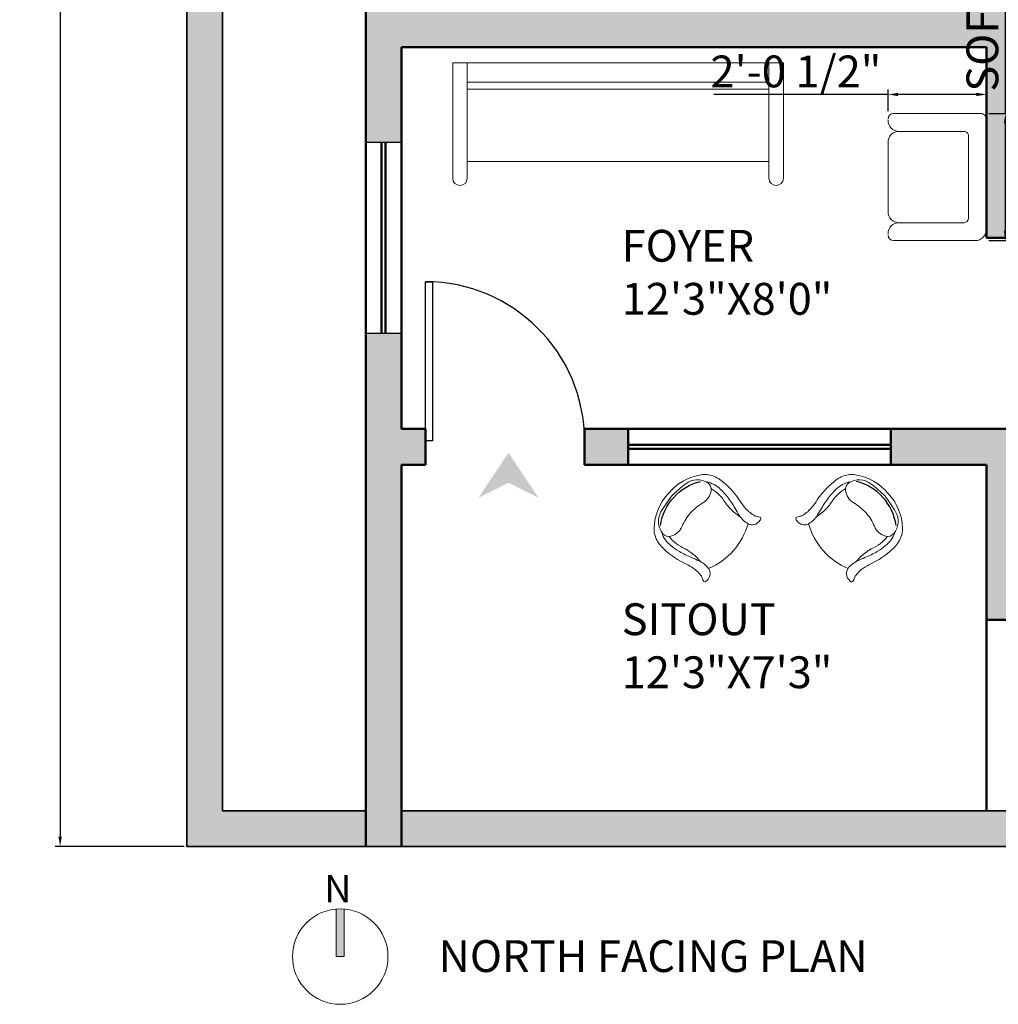
# Model space of a CAD drawing. Units: inches. Extents: x 2442 to 3851, y 589 to 2836.
# Tile 3 of 22: x 2452 to 2698, y 1362 to 1610. Entities that reach past the tile are written whole.
import ezdxf

# ---------------------------------------------------------------- set-up
doc = ezdxf.new("R2010")
doc.units = ezdxf.units.IN
for name, color, linetype, lineweight in [('A-ANNO-DIMS', 2, 'Continuous', 18), ('A-ANNO-SYMB', 1, 'Continuous', 18), ('A-ANNO-TEXT', 7, 'Continuous', 18), ('A-AREA-IDEN', 7, 'Continuous', 18), ('A-DOOR', 4, 'Continuous', 25), ('A-FURN', 8, 'Continuous', 18), ('A-GLAZ', 1, 'Continuous', 25), ('A-WALL', 7, 'Continuous', 50), ('A-WALL-PATT', 8, 'Continuous', 13), ('C-PROP', 7, 'Continuous', 35)]:
    doc.layers.add(name, color=color, linetype=linetype, lineweight=lineweight)
doc.layers.add('IFF-FURN-DETAIL', color=250, linetype='Continuous')
doc.styles.get("Standard").update_dxf_attribs({"font": 'arial.ttf'})
doc.dimstyles.new('ISO-25', dxfattribs={"dimtxt": 8, "dimasz": 2.5, "dimexe": 1.25, "dimexo": 0.625, "dimtad": 1, "dimlunit": 3, "dimtxsty": 'Standard', "dimcen": 2.5, "dimadec": 0, "dimazin": 0, "dimtfac": 1, "dimtmove": 0, "dimatfit": 3, "dimfxl": 1, "dimarcsym": 0})

# ---------------------------------------------------------------- blocks, each defined once
blk = doc.blocks.new('*U22')
for p, q in [((0, 0), (0, -6)), ((40, 0), (40, -6))]:
    blk.add_line(p, q)
blk.add_lwpolyline([(0, 0), (0, 40), (1.75, 40), (1.75, 0)], close=True)
blk.add_arc((0, 0), 40, 0, 90)
blk = doc.blocks.new('sofa-27')
at = {"color": 0, "linetype": 'ByBlock'}
for p, q in [((-0.0591, 0.0591), (-0.0591, 0.4902)), ((0.0945, 0.5198), (0.459, 0.5198)), ((0.6125, 0.0295), (0.6125, 0.4902)), ((0.0354, 0.1181), (0.0354, 0.4607)), ((0.518, 0.1181), (0.518, 0.4607)), ((0.4944, 0.0945), (0.0591, 0.0945)), ((0.583, 0), (0, 0))]:
    blk.add_line(p, q, dxfattribs=at)
for centre, radius, start, end in [((-0.0295, 0.4902), 0.0295, 90, 180), ((-0.0236, 0.4607), 0.0591, 360, 90), ((0.0945, 0.4607), 0.0591, 90, 180), ((0.459, 0.4607), 0.0591, 0, 90), ((0.5771, 0.4607), 0.0591, 90, 180), ((0.583, 0.4902), 0.0295, 0, 90), ((0.0591, 0.1181), 0.0236, 180, 270), ((0.4944, 0.1181), 0.0236, 270, 0), ((0, 0.0591), 0.0591, 180, 270), ((0.583, 0.0295), 0.0295, 270, 0)]:
    blk.add_arc(centre, radius, start, end, dxfattribs=at)
blk = doc.blocks.new('ILNG95')
for points in [[(120, 308, -0.32971), (51, 384, -0.036099), (50, 422, -0.497733), (75, 439, -0.070621), (96, 429, 0.101868), (133, 414, 0.091794), (259, 412, 0.024114), (351, 433, -0.090294), (638, 458, -0.132412), (775, 407, -0.068618), (816, 368, -0.184346), (943, 0, 1.803905)], [(120, 308, 0.138132), (244, 313, 0.001085), (325, 339, -0.034227), (462, 375, -0.033255), (567, 387, -0.137428), (727, 350, -4.561553)], [(120, 308, 0.138132), (244, 313, 0.001085), (325, 339, -0.034227), (462, 375, -0.033255), (567, 387, -0.137428), (727, 350, -4.561553)], [(235, 308, 0.064243), (394, 307, 0.04414), (433, 315, -0.118032), (643, 329, -6.296816)], [(235, 308, 0.064243), (394, 307, 0.04414), (433, 315, -0.118032), (643, 329, -6.296816)], [(639, 0, 0.078302), (612, 161, -0.233633), (633, 315, -0.28763), (710, 349, -0.317923), (875, 193, -0.032882), (900, 0, 1.140397)], [(639, 0, 0.078302), (612, 161, -0.233633), (633, 315, -0.28763), (710, 349, -0.317923), (875, 193, -0.032882), (900, 0, 1.140397)], [(120, -308, 0.32971), (51, -384, 0.036099), (50, -422, 0.497733), (75, -439, 0.070621), (96, -429, -0.101868), (133, -414, -0.091794), (259, -412, -0.024114), (351, -433, 0.090294), (638, -458, 0.132412), (775, -407, 0.068618), (816, -368, 0.184346), (943, 0, -1.803905)], [(639, 0, -0.078302), (612, -161, 0.233633), (633, -315, 0.28763), (710, -349, 0.317923), (875, -193, 0.032882), (900, 0, -1.140397)], [(639, 0, -0.078302), (612, -161, 0.233633), (633, -315, 0.28763), (710, -349, 0.317923), (875, -193, 0.032882), (900, 0, -1.140397)], [(120, -308, -0.138132), (244, -313, -0.001085), (325, -339, 0.034227), (462, -375, 0.033255), (567, -387, 0.137428), (727, -350, 4.561553)], [(120, -308, -0.138132), (244, -313, -0.001085), (325, -339, 0.034227), (462, -375, 0.033255), (567, -387, 0.137428), (727, -350, 4.561553)], [(235, -308, -0.064243), (394, -307, -0.04414), (433, -315, 0.118032), (643, -329, 6.296816)], [(235, -308, -0.064243), (394, -307, -0.04414), (433, -315, 0.118032), (643, -329, 6.296816)]]:
    blk.add_lwpolyline(points, format="xyb")
blk.add_arc((759, 1), 709, 154.3281, 205.801)
at = {"layer": 'IFF-FURN-DETAIL'}
blk.add_arc((326, -2), 549, 326.8997, 34.6691, dxfattribs=at)
blk.add_arc((326, -2), 549, 326.8997, 34.6691, dxfattribs=at)
blk = doc.blocks.new('*D32')
at = {"layer": 'A-ANNO-DIMS', "color": 0, "lineweight": -2, "transparency": 16777216}
for p, q in [((2492.97, 2001.86), (2460.53, 2001.86)), ((2461.78, 1999.36), (2461.78, 1404.36)), ((2492.97, 1401.86), (2460.53, 1401.86))]:
    blk.add_line(p, q, dxfattribs=at)
at = {"layer": 'A-ANNO-DIMS', "color": 0, "transparency": 16777216}
for points in [[(2461.36, 1999.36), (2462.2, 1999.36), (2461.78, 2001.86)], [(2461.36, 1404.36), (2462.2, 1404.36), (2461.78, 1401.86)]]:
    blk.add_solid(points, dxfattribs=at)
at = {"layer": 'Defpoints', "color": 0, "transparency": 16777216}
for p in [(2493.6, 2001.86), (2461.78, 1401.86), (2493.6, 1401.86)]:
    blk.add_point(p, dxfattribs=at)
at = {"layer": 'A-ANNO-DIMS', "color": 0, "transparency": 16777216, "insert": (2457.07, 1701.86), "char_height": 8, "attachment_point": 5, "rotation": 90}
blk.add_mtext("50'", dxfattribs=at)
blk = doc.blocks.new('SOFA-3SEAT')
for p, q in [((0, 29.02), (0, 0)), ((3.63, 0), (3.63, 29.02)), ((79.48, 29.02), (79.48, 0)), ((83.11, 29.02), (83.11, 0)), ((83.11, 0), (0, 0))]:
    blk.add_line(p, q)
for centre in [(1.81, 29.02), (81.3, 29.02)]:
    blk.add_arc(centre, 1.81, 0, 180)
blk = doc.blocks.new('NORTH-ARROW')
at = {"transparency": 33554687}
h = blk.add_hatch(color=256, dxfattribs=at)
h.dxf.hatch_style = 1
h.paths.add_polyline_path([(13, 12), (11, 12), (11, 23.96, -0.020861), (12, 24, -0.020861), (13, 23.96)])
for p, q in [((11, 24), (11, 12)), ((13, 12), (13, 23.96)), ((11, 12), (13, 12))]:
    blk.add_line(p, q)
blk.add_circle((12, 12), 12)
blk.add_text('N', height=6.9).set_placement((7.98, 25.6))
blk = doc.blocks.new('*D150')
at = {"layer": 'A-ANNO-DIMS', "color": 0, "lineweight": -2, "transparency": 16777216}
for p, q in [((2699.39, 1586.16), (2699.39, 1682.55)), ((2695.22, 1586.16), (2700.64, 1586.16)), ((2699.39, 1556.72), (2699.39, 1583.66)), ((2695.22, 1554.22), (2700.64, 1554.22))]:
    blk.add_line(p, q, dxfattribs=at)
at = {"layer": 'A-ANNO-DIMS', "color": 0, "transparency": 16777216}
for points in [[(2698.97, 1583.66), (2699.81, 1583.66), (2699.39, 1586.16)], [(2698.97, 1556.72), (2699.81, 1556.72), (2699.39, 1554.22)]]:
    blk.add_solid(points, dxfattribs=at)
at = {"layer": 'Defpoints', "color": 0, "transparency": 16777216}
for p in [(2694.6, 1586.16), (2699.39, 1586.16), (2694.6, 1554.22)]:
    blk.add_point(p, dxfattribs=at)
at = {"layer": 'A-ANNO-DIMS', "color": 0, "transparency": 16777216, "insert": (2694.63, 1635.61), "char_height": 8, "attachment_point": 5, "rotation": 90}
blk.add_mtext('SOFA CHAIR 2\'-8"', dxfattribs=at)
blk = doc.blocks.new('*D151')
at = {"layer": 'A-ANNO-DIMS', "color": 0, "lineweight": -2, "transparency": 16777216}
for p, q in [((2669.88, 1586.79), (2669.88, 1592.2)), ((2694.6, 1586.79), (2694.6, 1592.2)), ((2669.88, 1590.95), (2626.08, 1590.95)), ((2692.1, 1590.95), (2672.38, 1590.95))]:
    blk.add_line(p, q, dxfattribs=at)
at = {"layer": 'A-ANNO-DIMS', "color": 0, "transparency": 16777216}
for points in [[(2672.38, 1591.37), (2672.38, 1590.54), (2669.88, 1590.95)], [(2692.1, 1591.37), (2692.1, 1590.54), (2694.6, 1590.95)]]:
    blk.add_solid(points, dxfattribs=at)
at = {"layer": 'Defpoints', "color": 0, "transparency": 16777216}
for p in [(2669.88, 1590.95), (2669.88, 1586.16), (2694.6, 1586.16)]:
    blk.add_point(p, dxfattribs=at)
at = {"layer": 'A-ANNO-DIMS', "color": 0, "transparency": 16777216, "insert": (2646.73, 1595.71), "char_height": 8, "attachment_point": 5}
blk.add_mtext('2\'-0 1/2"', dxfattribs=at)

msp = doc.modelspace()

# ---------------------------------------------------------------- hatches: boundary and pattern name
at = {"layer": 'A-ANNO-SYMB'}
h = msp.add_hatch(color=256, dxfattribs=at)
h.dxf.hatch_style = 1
h.paths.add_polyline_path([(2574.486, 1500.868), (2566.935, 1489.543), (2574.486, 1493.318), (2582.036, 1489.543)])
at = {"layer": 'A-WALL-PATT'}
h = msp.add_hatch(color=256, dxfattribs=at)
h.dxf.hatch_style = 1
h.paths.add_polyline_path([(2502.599, 1992.864), (2719.571, 1992.864), (2719.687, 1994.649), (2720.167, 1997.319), (2721.479, 1992.864), (2726.325, 1992.864), (2727.448, 1994.93), (2729.005, 1997.153), (2728.372, 1992.864), (2728.871, 1992.864), (2730.114, 1994.505), (2731.833, 1996.09), (2730.966, 1993.206), (2730.864, 1992.864), (2771.772, 1992.864), (2771.887, 1994.649), (2772.368, 1997.319), (2773.68, 1992.864), (2778.526, 1992.864), (2779.649, 1994.93), (2781.206, 1997.153), (2780.572, 1992.864), (2781.072, 1992.864), (2782.315, 1994.505), (2784.034, 1996.09), (2783.167, 1993.206), (2783.065, 1992.864), (2821.282, 1992.864), (2821.398, 1994.649), (2821.878, 1997.319), (2823.19, 1992.864), (2828.036, 1992.864), (2829.159, 1994.93), (2830.716, 1997.153), (2830.083, 1992.864), (2830.582, 1992.864), (2831.825, 1994.505), (2833.544, 1996.09), (2832.677, 1993.206), (2832.575, 1992.864), (2869.287, 1992.864), (2869.403, 1994.649), (2869.884, 1997.319), (2871.195, 1992.864), (2876.042, 1992.864), (2877.165, 1994.93), (2878.721, 1997.153), (2878.088, 1992.864), (2878.587, 1992.864), (2879.83, 1994.505), (2881.55, 1996.09), (2880.682, 1993.206), (2880.58, 1992.864), (2919.335, 1992.864), (2919.451, 1994.649), (2919.932, 1997.319), (2921.243, 1992.864), (2926.09, 1992.864), (2927.213, 1994.93), (2928.77, 1997.153), (2928.136, 1992.864), (2928.635, 1992.864), (2929.878, 1994.505), (2931.598, 1996.09), (2930.73, 1993.206), (2930.628, 1992.864), (2966.155, 1992.864), (2966.27, 1994.649), (2966.751, 1997.319), (2968.063, 1992.864), (2972.909, 1992.864), (2974.032, 1994.93), (2975.589, 1997.153), (2974.955, 1992.864), (2975.455, 1992.864), (2976.698, 1994.505), (2978.417, 1996.09), (2977.55, 1993.206), (2977.448, 1992.864), (3010.53, 1992.864), (3010.646, 1994.649), (3011.127, 1997.319), (3012.438, 1992.864), (3017.285, 1992.864), (3018.408, 1994.93), (3019.964, 1997.153), (3019.331, 1992.864), (3019.83, 1992.864), (3021.073, 1994.505), (3022.793, 1996.09), (3021.925, 1993.206), (3021.823, 1992.864), (3057.996, 1992.864), (3058.45, 1995.382), (3059.191, 1992.864), (3065.64, 1992.864), (3067.287, 1995.216), (3066.94, 1992.864), (3068.717, 1992.864), (3070.116, 1994.153), (3069.728, 1992.864), (3084.599, 1992.864), (3084.599, 1983.791), (3085.291, 1983.828), (3084.599, 1983.434), (3084.599, 1932.114), (3085.291, 1932.151), (3084.599, 1931.757), (3084.599, 1886.278), (3085.291, 1886.315), (3084.599, 1885.921), (3084.599, 1410.864), (3066.599, 1410.864), (3066.599, 1401.864), (3093.599, 1401.864), (3093.599, 2001.864), (2493.599, 2001.864), (2493.599, 1401.864), (2538.599, 1401.864), (2538.599, 1410.864), (2502.599, 1410.864)])
h.paths.add_polyline_path([(2738.599, 1410.864), (2547.599, 1410.864), (2547.599, 1401.864), (2738.599, 1401.864)], flags=17)
h.paths.add_polyline_path([(2910.599, 1410.864), (2792.599, 1410.864), (2792.599, 1401.864), (2910.599, 1401.864), (2910.599, 1402.864)], flags=17)
h = msp.add_hatch(color=256, dxfattribs=at)
h.dxf.hatch_style = 1
h.paths.add_polyline_path([(2799.599, 1467.864), (2775.599, 1467.864), (2775.599, 1458.864), (2799.599, 1458.864)])
h.paths.add_polyline_path([(2703.599, 1506.864), (2670.599, 1506.864), (2670.599, 1497.864), (2694.599, 1497.864), (2694.599, 1458.864), (2733.599, 1458.864), (2733.599, 1467.864), (2709.417, 1467.864), (2703.599, 1467.864)])
h.paths.add_polyline_path([(2604.599, 1506.864), (2593.599, 1506.864), (2593.599, 1497.864), (2604.599, 1497.864)])
h.paths.add_polyline_path([(2547.599, 1497.864), (2553.599, 1497.864), (2553.599, 1506.864), (2547.599, 1506.864), (2547.599, 1530.864), (2538.599, 1530.864), (2538.599, 1401.864), (2547.599, 1401.864)])
h.paths.add_polyline_path([(2547.599, 1683.864), (2538.599, 1683.864), (2538.599, 1578.864), (2547.599, 1578.864), (2547.599, 1602.864), (2694.599, 1602.864), (2694.599, 1554.864), (2703.599, 1554.864), (2703.599, 1716.864), (2694.599, 1716.864), (2694.599, 1611.864), (2547.599, 1611.864)])
h.paths.add_polyline_path([(2892.599, 1497.864), (2883.599, 1497.864), (2883.599, 1488.228), (2883.599, 1467.864), (2865.599, 1467.864), (2865.599, 1458.864), (2892.599, 1458.864)])
h.paths.add_polyline_path([(3048.599, 1722.864), (3039.599, 1722.864), (3039.599, 1716.864), (2937.599, 1716.864), (2937.599, 1710.864), (3039.599, 1710.864), (3039.599, 1685.364), (3048.599, 1685.364)])
h.paths.add_polyline_path([(3048.599, 1779.864), (3039.599, 1779.864), (3039.599, 1773.864), (2961.599, 1773.864), (2961.599, 1791.864), (2955.599, 1791.864), (2955.599, 1773.864), (2895.599, 1773.864), (2895.599, 1821.864), (2916.599, 1821.864), (2916.599, 1827.864), (2889.599, 1827.864), (2889.599, 1773.864), (2886.599, 1773.864), (2886.599, 1764.864), (2937.599, 1764.864), (2937.599, 1746.864), (2943.599, 1746.864), (2943.599, 1764.864), (2956.06, 1764.864), (3039.599, 1764.864), (3039.599, 1758.864), (3048.599, 1758.864)])
h.paths.add_polyline_path([(3048.599, 1827.864), (2976.475, 1827.864, -0.1284593), (2975.705, 1827.665), (2964.694, 1827.687, -0.1198794), (2963.972, 1827.864), (2946.599, 1827.864), (2946.599, 1821.864), (3039.599, 1821.864), (3039.599, 1815.864), (3048.599, 1815.864)])
h.paths.add_polyline_path([(3048.599, 1956.864), (3023.366, 1956.864), (3023.277, 1956.402), (3023.088, 1956.864), (3019.494, 1956.864), (3019.543, 1955.479), (3019.146, 1956.864), (3015.599, 1956.864), (3015.599, 1947.864), (3039.599, 1947.864), (3039.599, 1875.864), (3048.599, 1875.864), (3048.599, 1880.743), (3047.576, 1881.614), (3046.081, 1883.417), (3044.931, 1885.453), (3047.541, 1883.949), (3048.599, 1883.343), (3048.599, 1910.588), (3047.049, 1909.235), (3047.896, 1910.862), (3048.599, 1911.909), (3048.599, 1918.826), (3042.477, 1917.032), (3043.928, 1918.154), (3045.59, 1919.165), (3047.525, 1920.009), (3048.599, 1920.305), (3048.599, 1926.579), (3047.576, 1927.45), (3046.081, 1929.252), (3044.931, 1931.289), (3047.541, 1929.785), (3048.599, 1929.179)])
h.paths.add_polyline_path([(2967.599, 1956.864), (2932.171, 1956.864), (2932.082, 1956.402), (2931.893, 1956.864), (2928.299, 1956.864), (2928.348, 1955.479), (2927.951, 1956.864), (2898.599, 1956.864), (2898.599, 1947.864), (2967.599, 1947.864)])
h.paths.add_polyline_path([(2850.599, 1956.864), (2834.118, 1956.864), (2834.029, 1956.402), (2833.84, 1956.864), (2830.245, 1956.864), (2830.294, 1955.479), (2829.897, 1956.864), (2796.599, 1956.864), (2796.599, 1947.864), (2799.599, 1947.864), (2838.599, 1947.864), (2838.599, 1827.864), (2835.599, 1827.864), (2835.599, 1824.864), (2835.599, 1818.864), (2838.599, 1818.864), (2838.599, 1764.864), (2850.599, 1764.864), (2850.599, 1770.864), (2850.599, 1773.864), (2847.599, 1773.864), (2847.599, 1947.864), (2850.599, 1947.864)])
h.paths.add_polyline_path([(2700.599, 1947.864), (2730.599, 1947.864), (2730.599, 1956.864), (2700.599, 1956.864), (2700.599, 1992.864), (2691.599, 1992.864), (2691.599, 1932.864), (2670.599, 1932.864), (2670.599, 1923.864), (2691.599, 1923.864), (2691.599, 1818.864), (2799.599, 1818.864), (2799.599, 1827.864), (2700.599, 1827.864)])
h.paths.add_polyline_path([(2640.599, 1932.864), (2538.599, 1932.864), (2538.599, 1868.364), (2547.599, 1868.364), (2547.599, 1923.864), (2640.599, 1923.864), (2640.599, 1929.864)])
h.paths.add_polyline_path([(2547.599, 1820.364), (2538.599, 1820.364), (2538.599, 1731.864), (2547.599, 1731.864), (2547.599, 1755.864), (2694.599, 1755.864), (2694.599, 1752.864), (2697.599, 1752.864), (2703.599, 1752.864), (2703.599, 1764.864), (2547.599, 1764.864)])
h.paths.add_polyline_path([(2725.858, 1838.187), (2790.115, 1838.187), (2790.115, 1868.602), (2725.858, 1868.602)], flags=25)
h.paths.add_polyline_path([(2892.599, 1671.864), (2883.599, 1671.864), (2883.599, 1563.864), (2892.599, 1563.864), (2892.599, 1602.864), (3048.599, 1602.864), (3048.599, 1637.364), (3039.599, 1637.364), (3039.599, 1611.864), (2892.599, 1611.864)])

# ---------------------------------------------------------------- linework, layer by layer
at = {"layer": 'A-FURN'}
for p, q in [((2564.096, 1594.07), (2639.951, 1594.07)), ((2564.096, 1592.257), (2639.951, 1592.257)), ((2639.951, 1574.118), (2564.096, 1574.118))]:
    msp.add_line(p, q, dxfattribs=at)
at = {"layer": 'A-GLAZ'}
for p, q in [((2547.599, 1578.864), (2538.599, 1578.864)), ((2547.599, 1530.864), (2538.599, 1530.864))]:
    msp.add_line(p, q, dxfattribs=at)
at = {"layer": 'A-WALL'}
for p, q in [((2538.599, 1992.864), (2538.599, 1401.864)), ((2547.599, 1602.864), (2694.599, 1602.864)), ((2547.599, 1602.864), (2547.599, 1506.864)), ((2694.599, 1554.864), (2694.599, 1602.864)), ((2542.599, 1578.864), (2542.599, 1530.864)), ((2543.599, 1578.864), (2543.599, 1530.864)), ((2694.599, 1554.864), (2703.599, 1554.864)), ((2547.599, 1506.864), (2553.599, 1506.864)), ((2553.599, 1506.864), (2553.599, 1497.864)), ((2593.599, 1506.864), (2593.599, 1497.864)), ((2593.599, 1506.864), (2703.599, 1506.864)), ((2604.599, 1497.864), (2604.599, 1506.864)), ((2670.599, 1497.864), (2670.599, 1506.864)), ((2604.599, 1502.864), (2670.599, 1502.864)), ((2604.599, 1501.864), (2670.599, 1501.864)), ((2547.599, 1497.864), (2553.599, 1497.864)), ((2547.599, 1497.864), (2547.599, 1401.864)), ((2593.599, 1497.864), (2694.599, 1497.864)), ((2694.599, 1410.864), (2694.599, 1497.864)), ((2694.599, 1458.864), (2892.599, 1458.864))]:
    msp.add_line(p, q, dxfattribs=at)
at = {"layer": 'C-PROP'}
for points in [[(3066.599, 1401.864), (3093.599, 1401.864), (3093.599, 2001.864), (2493.599, 2001.864), (2493.599, 1401.864), (2738.599, 1401.864)], [(3066.599, 1410.864), (3084.599, 1410.864), (3084.599, 1992.864), (2502.599, 1992.864), (2502.599, 1410.864), (2538.599, 1410.864)], [(2547.599, 1410.864), (2738.599, 1410.864)]]:
    msp.add_lwpolyline(points, dxfattribs=at)

# ---------------------------------------------------------------- block references
at = {"layer": 'A-ANNO-SYMB'}
msp.add_blockref('NORTH-ARROW', (2520.188, 1362.181), dxfattribs=at)
at = {"layer": 'A-DOOR'}
msp.add_blockref('*U22', (2553.599, 1503.864), dxfattribs=at)
at = {"layer": 'A-FURN', "rotation": 180}
msp.add_blockref('SOFA-3SEAT', (2643.579, 1598.905), dxfattribs=at)
at = {"layer": 'A-FURN'}
for name, p, xscale, yscale, zscale, rotation in [('sofa-27', (2694.599, 1557.029), 47.56239266872987, 47.56239266872987, 47.56239266872987, 89.9999999999668), ('ILNG95', (2631.917, 1475.449), -0.0243705291132055, 0.0243705291132055, 0.0243705291132055, 318.5881218623716), ('ILNG95', (2652.675, 1475.449), 0.0243705291132055, 0.0243705291132055, 0.0243705291132055, 41.41187813762839)]:
    msp.add_blockref(name, p, dxfattribs=dict(at, xscale=xscale, yscale=yscale, zscale=zscale, rotation=rotation))

# ---------------------------------------------------------------- texts
at = {"layer": 'A-ANNO-TEXT', "insert": (2556.881, 1378.304), "char_height": 8, "attachment_point": 1}
msp.add_mtext_dynamic_manual_height_columns('{\\fTimes New Roman|b0|i0|c0|p18;NORTH FACING PLAN}', width=196.26071, gutter_width=12.5, heights=[0], dxfattribs=at)
at = {"layer": 'A-AREA-IDEN', "char_height": 8, "attachment_point": 1}
for s, insert in [('{\\fTimes New Roman|b0|i0|c0|p18;FOYER\\P12\'3"X8\'0"}', (2602.937, 1556.905)), ('{\\fTimes New Roman|b0|i0|c0|p18;SITOUT\\P12\'3"X7\'3"}', (2602.937, 1463.006))]:
    msp.add_mtext_dynamic_manual_height_columns(s, width=110.76054, gutter_width=12.5, heights=[0], dxfattribs=dict(at, insert=insert))

# ---------------------------------------------------------------- dimensions: what is measured, and where the dimension line sits
at = {"layer": 'A-ANNO-DIMS'}
for base, p1, p2, angle, override, picture, middle in [((2461.781, 1401.864), (2493.599, 2001.864), (2493.599, 1401.864), 90, {"dimclrd": 0, "dimclre": 0, "dimclrt": 0}, '*D32', (2457.071, 1701.864)), ((2669.878, 1590.953), (2694.599, 1586.162), (2669.878, 1586.162), 180, {"dimdec": 1, "dimrnd": 0, "dimzin": 1, "dimlunit": 4, "dimfrac": 2}, '*D151', (2646.731, 1595.715))]:
    dim = msp.add_linear_dim(base=base, p1=p1, p2=p2, angle=angle, dimstyle='ISO-25', override=override, dxfattribs=at)
    dim.commit()
    dim.dimension.update_dxf_attribs({"geometry": picture, "text_midpoint": middle})
dim = msp.add_linear_dim(base=(2699.39, 1586.162), p1=(2694.599, 1554.22), p2=(2694.599, 1586.162), angle=90, text='SOFA CHAIR <>', dimstyle='ISO-25', override={"dimdec": 1, "dimrnd": 0, "dimzin": 1, "dimlunit": 4, "dimfrac": 2}, dxfattribs=at)
dim.commit()
dim.dimension.update_dxf_attribs({"geometry": '*D150', "text_midpoint": (2694.626, 1635.606)})

doc.saveas('drawing.dxf')
